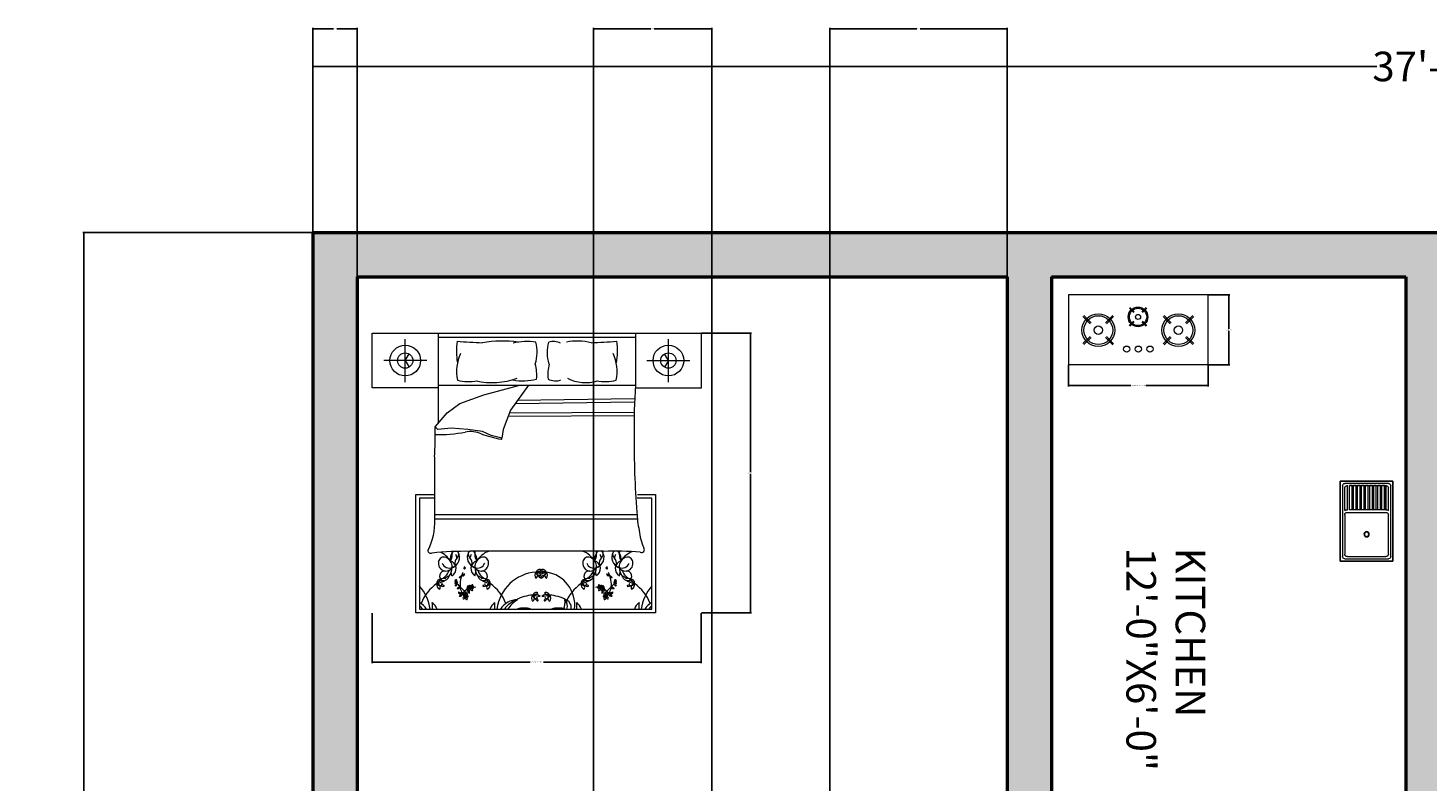
# Model space of a CAD drawing. Units: inches. Extents: x -17 to 536, y -817 to 53.
# Tile 6 of 9: x -17 to 268, y -100 to 53. Entities that reach past the tile are written whole.
import ezdxf

# ---------------------------------------------------------------- set-up
doc = ezdxf.new("R2010")
doc.units = ezdxf.units.IN
doc.header["$MEASUREMENT"] = 0
for name, color, linetype, lineweight in [('A-ANNO-DIMS', 2, 'Continuous', 18), ('A-AREA-IDEN', 7, 'Continuous', 18), ('A-EQPM', 8, 'Continuous', 18), ('A-FLOR-FIXT', 9, 'Continuous', 18), ('A-FURN', 8, 'Continuous', 13), ('A-WALL', 7, 'Continuous', 50), ('A-WALL-PATT', 22, 'Continuous', 13)]:
    doc.layers.add(name, color=color, linetype=linetype, lineweight=lineweight)
doc.styles.get("Standard").update_dxf_attribs({"font": 'arial.ttf'})
doc.dimstyles.get("Standard").update_dxf_attribs({"dimtxt": 0.18, "dimasz": 0.18, "dimexe": 0.18, "dimexo": 0.0625, "dimgap": 0.09, "dimtad": 0, "dimtih": 1, "dimtoh": 1, "dimdec": 0, "dimzin": 0, "dimdsep": 46, "dimlunit": 3, "dimtxsty": 'Standard', "dimcen": 0.09, "dimadec": 0, "dimazin": 0, "dimtfac": 1, "dimtdec": 0, "dimtofl": 0, "dimtmove": 0, "dimatfit": 3, "dimfxl": 1, "dimtolj": 1, "dimtzin": 0, "dimarcsym": 0})

# ---------------------------------------------------------------- blocks, each defined once
blk = doc.blocks.new('*D1')
at = {"layer": 'A-ANNO-DIMS', "color": 0, "lineweight": -2, "transparency": 16777216}
for p, q in [((41.37, 11.61), (41.37, 45.45)), ((41.55, 45.27), (257.47, 45.27)), ((494.19, 45.27), (278.26, 45.27)), ((494.37, 11.61), (494.37, 45.45))]:
    blk.add_line(p, q, dxfattribs=at)
at = {"layer": 'A-ANNO-DIMS', "color": 0, "transparency": 16777216}
for points in [[(41.55, 45.3), (41.55, 45.24), (41.37, 45.27)], [(494.19, 45.3), (494.19, 45.24), (494.37, 45.27)]]:
    blk.add_solid(points, dxfattribs=at)
at = {"layer": 'Defpoints', "color": 0, "transparency": 16777216}
for p in [(494.37, 45.27), (41.37, 11.55), (494.37, 11.55)]:
    blk.add_point(p, dxfattribs=at)
at = {"layer": 'A-ANNO-DIMS', "color": 0, "transparency": 16777216, "insert": (267.87, 45.27), "char_height": 6, "attachment_point": 5}
blk.add_mtext('\\A1;37\'-9"', dxfattribs=at)
blk = doc.blocks.new('*D2')
at = {"layer": 'A-ANNO-DIMS', "color": 0, "lineweight": -2, "transparency": 16777216}
for p, q in [((41.3, 11.55), (-5.38, 11.55)), ((-5.2, 11.37), (-5.2, -378.8)), ((-5.2, -775.27), (-5.2, -385.1)), ((41.3, -775.45), (-5.38, -775.45))]:
    blk.add_line(p, q, dxfattribs=at)
at = {"layer": 'A-ANNO-DIMS', "color": 0, "transparency": 16777216}
for points in [[(-5.23, 11.37), (-5.17, 11.37), (-5.2, 11.55)], [(-5.23, -775.27), (-5.17, -775.27), (-5.2, -775.45)]]:
    blk.add_solid(points, dxfattribs=at)
at = {"layer": 'Defpoints', "color": 0, "transparency": 16777216}
for p in [(41.37, 11.55), (-5.2, -775.45), (41.37, -775.45)]:
    blk.add_point(p, dxfattribs=at)
at = {"layer": 'A-ANNO-DIMS', "color": 0, "transparency": 16777216, "insert": (-5.2, -381.95), "char_height": 6, "attachment_point": 5}
blk.add_mtext('\\A1;65\'-7"', dxfattribs=at)
blk = doc.blocks.new('М12 540х820')
for p, q in [((0, 540), (-820, 540)), ((-820, 540), (-820, 0)), ((-798, 495), (-798, 45)), ((-45, 517), (-775, 517)), ((-775, 468), (-775, 72)), ((-348, 495), (-748, 495)), ((-320, 468), (-320, 72)), ((-302, 495), (-65, 495)), ((-294, 468), (-294, 472)), ((-294, 468), (-45, 468)), ((-294, 447), (-45, 447)), ((-294, 420), (-294, 447)), ((-45, 470), (-45, 468)), ((-45, 420), (-45, 447)), ((-22, 45), (-22, 495)), ((0, 0), (0, 540)), ((-294, 420), (-45, 420)), ((-294, 405), (-45, 405)), ((-294, 378), (-294, 405)), ((-294, 378), (-45, 378)), ((-294, 336), (-294, 363)), ((-294, 363), (-45, 363)), ((-294, 336), (-45, 336)), ((-294, 295), (-294, 322)), ((-294, 322), (-45, 322)), ((-294, 295), (-45, 295)), ((-45, 378), (-45, 405)), ((-45, 336), (-45, 363)), ((-45, 295), (-45, 322)), ((-294, 253), (-294, 280)), ((-294, 280), (-45, 280)), ((-294, 253), (-45, 253)), ((-294, 211), (-294, 238)), ((-294, 238), (-45, 238)), ((-294, 211), (-45, 211)), ((-294, 170), (-294, 197)), ((-294, 197), (-45, 197)), ((-294, 170), (-45, 170)), ((-294, 128), (-294, 155)), ((-294, 155), (-45, 155)), ((-45, 253), (-45, 280)), ((-45, 211), (-45, 238)), ((-45, 170), (-45, 197)), ((-45, 128), (-45, 155)), ((-820, 0), (0, 0)), ((-775, 22), (-45, 22)), ((-748, 45), (-348, 45)), ((-302, 45), (-65, 45)), ((-294, 128), (-45, 128)), ((-294, 114), (-45, 114)), ((-294, 87), (-294, 114)), ((-294, 87), (-45, 87)), ((-294, 72), (-45, 72)), ((-45, 87), (-45, 114)), ((-45, 70), (-45, 72))]:
    blk.add_line(p, q)
at = {"ltscale": 0.06}
for p, q in [((-820, 0), (-820, 540)), ((-820, 540), (0, 540)), ((-294, 447), (-45, 447)), ((-294, 405), (-294, 447)), ((-45, 447), (-45, 420)), ((0, 540), (0, 537)), ((0, 537), (0, 0)), ((-294, 363), (-294, 405)), ((-294, 322), (-294, 363)), ((-294, 280), (-294, 322)), ((-45, 420), (-45, 378)), ((-45, 378), (-45, 336)), ((-45, 336), (-45, 295)), ((-45, 295), (-45, 253)), ((-294, 238), (-294, 280)), ((-294, 197), (-294, 238)), ((-294, 155), (-294, 197)), ((-294, 114), (-294, 155)), ((-45, 253), (-45, 211)), ((-45, 211), (-45, 170)), ((-45, 170), (-45, 128)), ((0, 0), (-820, 0)), ((-294, 72), (-294, 114)), ((-45, 72), (-294, 72)), ((-45, 128), (-45, 87)), ((-45, 87), (-45, 72))]:
    blk.add_line(p, q, dxfattribs=at)
at = {"extrusion": (0, 0, -1)}
for centre, major_axis, start_param, end_param in [((-775, 495), (-15.9, 15.9), -0.785398, 0.785398), ((-775, 495), (-15.9, 15.9), -0.785398, 0.785398), ((-748, 468), (-19.1, -19.1), 0.785398, 2.356194), ((-748, 468), (-19.1, -19.1), 0.785398, 2.356194), ((-348, 468), (-19.1, 19.1), 0.785398, 2.356194), ((-348, 468), (-19.1, 19.1), 0.785398, 2.356194), ((-343, 468), (-35, 35), 1.779263, 2.356194), ((-343, 468), (-35, 35), 1.779263, 2.356192), ((-343, 468), (-35, 35), 2.356192, 2.356194), ((-72, 469), (-19.3, 19.3), 1.0328, 2.38382), ((-72, 469), (-19.3, 19.3), 1.0328, 1.064673), ((-72, 469), (-19.3, 19.3), 1.064673, 2.328569), ((-45, 495), (-15.9, -15.9), 2.356194, 3.926991), ((-45, 495), (-15.9, -15.9), 2.356194, 3.926991), ((-72, 469), (-19.3, 19.3), 2.328569, 2.38382), ((-545, 270), (-19.1, -19.1), 3.926991, 10.210176), ((-545, 270), (-19.1, -19.1), 3.926991, 10.210176), ((-545, 270), (-15.9, -15.9), 3.926991, 10.210176), ((-545, 270), (-15.9, -15.9), 3.926991, 10.210176), ((-775, 45), (-15.9, -15.9), 5.497787, 7.068583), ((-775, 45), (-15.9, -15.9), 5.497787, 7.068583), ((-748, 72), (-19.1, 19.1), 3.926991, 5.497787), ((-748, 72), (-19.1, 19.1), 3.926991, 5.497787), ((-348, 72), (-19.1, -19.1), 3.926991, 5.497787), ((-348, 72), (-19.1, -19.1), 3.926991, 5.497787), ((-343, 72), (-35, -35), 3.926991, 4.503922), ((-343, 72), (-35, -35), 3.926991, 4.503922), ((-72, 71), (-19.3, -19.3), 3.899365, 5.250385), ((-72, 71), (-19.3, -19.3), 5.218512, 5.250385), ((-72, 71), (-19.3, -19.3), 3.954617, 5.218512), ((-72, 71), (-19.3, -19.3), 3.899365, 3.954617), ((-45, 45), (-15.9, 15.9), 2.356194, 3.926991), ((-45, 45), (-15.9, 15.9), 2.356194, 3.926991)]:
    blk.add_ellipse(centre, major_axis=major_axis, ratio=1, start_param=start_param, end_param=end_param, dxfattribs=at)
blk = doc.blocks.new('BED-WITH-NIGHTSTANDS-COMPACT')
for p, q in [((0, 56.83), (66.83, 56.83)), ((6.68, 46.9), (6.68, 55.63)), ((13.37, 56.83), (13.37, 38.49)), ((53.46, 55.97), (13.37, 55.97)), ((60.14, 46.9), (60.14, 55.63)), ((11.05, 51.26), (2.32, 51.26)), ((55.78, 51.26), (64.51, 51.26)), ((13.37, 46.27), (53.46, 46.27)), ((22.65, 44.28), (29.94, 46.27)), ((31.72, 46.27), (28.06, 41.17)), ((17.78, 42.53), (22.65, 44.28)), ((53.26, 42.81), (28.99, 42.47)), ((53.28, 43.49), (29.49, 43.16)), ((12.77, 37.79), (15.2, 40.63)), ((15.2, 40.63), (17.78, 42.53)), ((28.06, 41.17), (26.57, 37.25)), ((53.23, 40.02), (27.58, 39.91)), ((53.22, 40.7), (27.85, 40.6)), ((13.31, 37.25), (12.77, 37.79)), ((16.02, 37.52), (13.31, 37.25)), ((19.4, 37.25), (16.02, 37.52)), ((22.38, 36.85), (19.4, 37.25)), ((26.57, 37.25), (26.3, 35.49)), ((24.14, 36.03), (22.38, 36.85)), ((26.3, 35.49), (24.14, 36.03)), ((8.82, 24.07), (12.6, 24.07)), ((8.82, 0), (8.82, 24.07)), ((12.6, 23.3), (9.59, 23.3)), ((9.59, 23.3), (9.59, 0.77)), ((56.77, 23.3), (53.82, 23.3)), ((53.83, 24.07), (57.54, 24.07)), ((56.77, 0.77), (56.77, 23.3)), ((57.54, 24.07), (57.54, 0)), ((53.77, 19.9), (12.6, 19.9)), ((53.83, 19.07), (12.6, 19.07)), ((46.98, 12.51), (19.85, 12.51)), ((16.18, 7.55), (16.03, 8.3)), ((20.85, 7.55), (21, 8.3)), ((45.51, 7.55), (45.36, 8.3)), ((50.18, 7.55), (50.33, 8.3)), ((9.59, 0.77), (56.77, 0.77)), ((57.54, 0), (8.82, 0))]:
    blk.add_line(p, q)
for points in [[(13.37, 45.69), (0, 45.69), (0, 56.83)], [(53.46, 56.83), (53.46, 45.69), (66.83, 45.69), (66.83, 56.83)], [(6.68, 51.26), (7.46, 52.61)], [(6.68, 51.26), (7.46, 49.91)], [(60.14, 51.26), (59.36, 52.61)], [(60.14, 51.26), (59.36, 49.91)]]:
    blk.add_lwpolyline(points)
for points in [[(17.2, 55.17, 0.074897), (17.28, 50.8, -0.472817)], [(33.1, 50.56, 0.14099), (33.23, 55.01, 0.235245)], [(35.95, 50.56, -0.14099), (35.82, 55.01, -0.235245)], [(49.62, 55.17, -0.074897), (49.54, 50.8, 0.472817)], [(12.63, 31.67, 0.001242), (12.6, 18.99, -0.127202), (11.26, 12.67)], [(53.75, 20.43, 0.056112), (54.23, 16.75, 0.095341), (55.17, 13.21)]]:
    blk.add_lwpolyline(points, format="xyb")
for centre, radius in [((6.68, 51.26), 3.12), ((60.14, 51.26), 3.12), ((6.68, 51.26), 1.56), ((60.14, 51.26), 1.56), ((18.93, 3.33), 0.17), ((20.04, 5.13), 0.17), ((46.32, 5.13), 0.17), ((47.43, 3.33), 0.17)]:
    blk.add_circle(centre, radius)
for centre, radius, start, end in [((54.04, 691.14), 637.04, 266.68521, 267.14978), ((26.36, 30.98), 24.24, 82.2196, 99.497), ((31.48, 43.23), 11.91, 81.5249, 103.96), ((36.74, 51.83), 3.31, 63.3437, 106.1026), ((41.69, 43.47), 11.75, 76.3427, 101.1841), ((12.79, 691.14), 637.04, 272.85022, 273.31479), ((25.72, 49.05), 8.61, 155.1316, 191.7583), ((41.11, 49.05), 8.61, 348.2417, 24.8684), ((25.22, 48.32), 8.19, 354.0129, 15.8293), ((43.83, 48.32), 8.19, 164.1707, 185.9871), ((19.59, 55.95), 8.96, 255.1039, 281.0369), ((24.3, 62.31), 15.53, 258.0397, 289.2615), ((30.59, 58.92), 11.78, 259.8617, 283.6238), ((37.18, 50.68), 3.54, 245.0183, 288.5407), ((43.37, 55.29), 8.51, 243.8761, 286.1746), ((47.24, 55.95), 8.96, 258.9631, 284.8961), ((173.26, 38.1), 120.08, 176.1, 180.9282), ((-48.51, 36.13), 61.3, 355.8294, 1.553), ((13.91, 61.46), 25.22, 267.4519, 281.3392), ((19.94, 31.39), 5.44, 66.2616, 101.3392), ((30.94, 60.75), 25.92, 250.1194, 259.3383), ((26.15, 35.44), 0.161, 268.8623, 19.7536), ((209.82, 33.74), 156.63, 179.1145, 184.8735), ((11.87, 12.72), 0.617, 183.98, 297.3412), ((19.05, -57.06), 69.57, 89.3433, 95.6887), ((11.61, 7.8), 5.06, 33.6671, 63.2997), ((18.39, 10.81), 2.58, 145.785, 184.7304), ((13.47, 12.01), 2.77, 328.8218, 9.1554), ((16.89, 11.77), 0.805, 120.0293, 142.325), ((15.61, 11.29), 2.13, 289.2822, 29.1751), ((15.29, 10.91), 1.92, 7.436, 29.9149), ((16.55, 11.93), 1, 311.5653, 23.8354), ((16.89, 11.77), 0.805, 44.4517, 63.558), ((21.42, 11.29), 2.13, 150.8249, 250.7178), ((20.48, 11.93), 1, 156.1646, 228.4347), ((20.14, 11.77), 0.805, 113.229, 135.5483), ((21.74, 10.91), 1.92, 150.0851, 172.564), ((20.14, 11.77), 0.805, 37.675, 66.7144), ((18.64, 10.81), 2.58, 355.2696, 34.215), ((23.57, 12.01), 2.77, 169.7133, 211.1782), ((25.42, 7.8), 5.06, 111.4941, 146.3329), ((40.94, 7.8), 5.06, 33.6671, 68.5059), ((47.72, 10.81), 2.58, 145.785, 184.7304), ((42.79, 12.01), 2.77, 328.8218, 10.2867), ((46.22, 11.77), 0.805, 113.2856, 142.325), ((44.94, 11.29), 2.13, 289.2822, 29.1751), ((44.62, 10.91), 1.92, 7.436, 29.9149), ((46.22, 11.77), 0.805, 44.4517, 66.7144), ((45.88, 11.93), 1, 311.5653, 23.8354), ((49.03, -52.49), 65.03, 85.2402, 91.8035), ((50.75, 11.29), 2.13, 150.8249, 250.7178), ((49.81, 11.93), 1, 156.1646, 228.4347), ((49.47, 11.77), 0.805, 106.6343, 135.5483), ((51.07, 10.91), 1.92, 150.0851, 172.564), ((49.47, 11.77), 0.805, 37.675, 72.5814), ((47.97, 10.81), 2.58, 355.2696, 34.215), ((52.9, 12.01), 2.77, 169.249, 211.1782), ((54.75, 7.8), 5.06, 113.6453, 146.3329), ((54.66, 12.87), 0.609, 246.5219, 33.8264), ((15.02, 10.07), 1.6, 174.9449, 262.8857), ((14.56, 10.23), 1.13, 84.4856, 181.0538), ((15.65, 10.67), 1.55, 201.5819, 291.4221), ((12.66, 9.7), 3.15, 301.2614, 341.7045), ((14.21, 9.39), 2.01, 355.2933, 76.921), ((14.74, 10.42), 1.94, 272.3591, 324.0401), ((12.63, 9.45), 3.59, 326.2883, 356.5076), ((15.35, 8.99), 1.66, 299.9085, 73.1337), ((18.39, 10.81), 2.58, 212.7011, 216.3445), ((16.4, 9.69), 0.415, 257.3041, 15.1471), ((18.13, 10.15), 1.37, 131.5653, 195.1471), ((18.71, 9.06), 0.129, 102.7051, 280.4384), ((18.69, 9.14), 0.209, 280.4384, 100.4136), ((18.9, 10.15), 1.37, 344.8529, 48.4347), ((21.68, 8.99), 1.66, 106.8663, 240.0915), ((20.63, 9.69), 0.415, 164.8529, 282.6959), ((18.64, 10.81), 2.58, 323.6555, 327.2989), ((22.29, 10.42), 1.94, 215.9599, 267.6409), ((22.82, 9.39), 2.01, 103.079, 184.7067), ((21.38, 10.67), 1.55, 248.5779, 338.4181), ((24.4, 9.45), 3.59, 183.4924, 213.7117), ((24.37, 9.7), 3.15, 198.2955, 238.7386), ((22.01, 10.07), 1.6, 277.1143, 5.0551), ((22.47, 10.23), 1.13, 358.9462, 95.5144), ((33.95, 8.1), 0.723, 63.0274, 163.8037), ((33.22, 9.79), 1.49, 271.4585, 315.3727), ((34.64, 8.1), 0.723, 16.1963, 116.9726), ((35.37, 9.79), 1.49, 224.6273, 268.5415), ((44.35, 10.07), 1.6, 174.9449, 262.8857), ((43.89, 10.23), 1.13, 84.4856, 181.0538), ((44.98, 10.67), 1.55, 201.5819, 291.4221), ((41.99, 9.7), 3.15, 301.2614, 341.7045), ((43.54, 9.39), 2.01, 355.2933, 76.921), ((44.07, 10.42), 1.94, 272.3591, 324.0401), ((41.96, 9.45), 3.59, 326.2883, 356.5076), ((44.68, 8.99), 1.66, 299.9085, 73.1337), ((47.72, 10.81), 2.58, 212.7011, 216.3445), ((45.73, 9.69), 0.415, 257.3041, 15.1471), ((47.46, 10.15), 1.37, 131.5653, 195.1471), ((47.67, 9.14), 0.209, 79.5864, 259.5616), ((47.65, 9.06), 0.129, 259.5616, 77.2949), ((48.23, 10.15), 1.37, 344.8529, 48.4347), ((51.01, 8.99), 1.66, 106.8663, 240.0915), ((49.96, 9.69), 0.415, 164.8529, 282.6959), ((47.97, 10.81), 2.58, 323.6555, 327.2989), ((51.62, 10.42), 1.94, 215.9599, 267.6409), ((52.15, 9.39), 2.01, 103.079, 184.7067), ((50.71, 10.67), 1.55, 248.5779, 338.4181), ((53.73, 9.45), 3.59, 183.4924, 213.7117), ((53.7, 9.7), 3.15, 198.2955, 238.7386), ((51.34, 10.07), 1.6, 277.1143, 5.0551), ((51.8, 10.23), 1.13, 358.9462, 95.5144), ((18.03, -1.26), 8.73, 124.3865, 158.5908), ((13.8, 6.11), 0.723, 92.9516, 193.728), ((14.05, 5.73), 0.968, 167.7115, 249.0387), ((12.32, 7.21), 1.49, 301.3827, 345.2969), ((14.22, 5.13), 1.38, 75.4653, 144.2343), ((11.78, 11.9), 6.1, 282.5173, 297.1824), ((13.08, 5.21), 0.729, 328.4633, 88.2869), ((14.55, 7.6), 2.21, 228.8402, 267.9352), ((13.73, 6.27), 0.714, 207.6827, 313.7762), ((14.65, 7.5), 1, 80.264, 250.8688), ((14.45, 6.41), 0.615, 63.9755, 143.2681), ((14.16, 5.82), 0.0944, 313.7762, 249.7183), ((14.41, 7.8), 1.25, 265.969, 344.3045), ((15.76, 6.13), 1.33, 96.1662, 141.5825), ((16.98, 6.4), 0.284, 101.5637, 142.6358), ((16.74, 6.14), 0.17, 273.2768, 86.7232), ((16.94, 6.3), 0.163, 91.1081, 181.8675), ((17.28, 6.2), 0.517, 203.4276, 227.6104), ((17.11, 5.97), 0.352, 80.3487, 133.6538), ((17.05, 6.26), 0.278, 229.7889, 317.6792), ((16.75, 6.63), 0.409, 288.7263, 352.5032), ((16.74, 5.67), 0.395, 355.053, 68.3618), ((17.05, 5.61), 0.557, 83.0852, 105.7171), ((17.03, 6.61), 0.131, 345.2356, 144.9248), ((13.19, 0.99), 6.35, 43.1541, 52.0459), ((17.15, 6.18), 0.147, 317.6792, 80.3487), ((17.97, 7.07), 0.351, 101.3256, 154.4621), ((17.46, 8.26), 1.06, 280.2588, 300.656), ((17.71, 9.1), 1.88, 268.3264, 277.1302), ((23.34, 5.69), 5.53, 163.5842, 183.8277), ((17.24, 8.26), 1.07, 308.2101, 316.3071), ((17.9, 7.55), 0.321, 278.3432, 4.2869), ((17.72, 7.83), 0.56, 300.656, 332.6341), ((18.14, 7.46), 0.136, 55.7657, 157.4417), ((23.34, 5.69), 5.53, 153.0032, 159.8941), ((18.35, 7.59), 0.136, 84.3784, 186.0543), ((18.22, 8.13), 0.56, 269.1859, 301.164), ((18.39, 7.84), 0.321, 237.5332, 323.4768), ((18.08, 8.76), 1.07, 285.5129, 293.6099), ((17.97, 8.56), 1.06, 301.164, 321.5612), ((18.78, 7.55), 0.351, 87.3579, 140.4944), ((17.11, 8.74), 1.88, 324.6898, 333.4936), ((20.33, 5.59), 0.131, 345.2356, 144.9248), ((21.27, 6.13), 1.33, 38.4175, 83.8338), ((22.62, 7.8), 1.25, 195.6955, 274.031), ((22.38, 7.5), 1, 289.1312, 99.736), ((22.59, 6.41), 0.615, 36.7319, 116.0245), ((22.81, 5.13), 1.38, 35.7657, 104.5347), ((25.25, 11.9), 6.1, 242.8176, 257.4827), ((22.48, 7.6), 2.21, 272.0648, 311.1598), ((23.3, 6.27), 0.714, 226.2238, 332.3173), ((22.88, 5.86), 0.0569, 290.2667, 226.2271), ((23.95, 5.21), 0.729, 91.7131, 211.5367), ((23.23, 6.11), 0.723, 346.272, 87.0484), ((24.71, 7.21), 1.49, 194.7031, 238.6173), ((22.99, 5.73), 0.968, 290.9613, 12.2885), ((19, -1.26), 8.73, 21.4092, 55.6135), ((33.93, -0.4), 8.73, 94.4623, 172.255), ((33.97, 7.65), 0.968, 137.7873, 219.1145), ((32.87, 7.68), 0.729, 298.5391, 58.3627), ((33.82, 7.04), 1.38, 45.5411, 114.3101), ((35.08, 14.12), 6.1, 252.593, 267.2582), ((33.97, 8.27), 0.714, 177.7585, 283.852), ((35.34, 9.01), 2.21, 198.9159, 238.011), ((34.77, 7.04), 1.38, 65.6899, 134.4589), ((33.51, 14.12), 6.1, 272.7418, 287.407), ((34.12, 7.67), 0.0944, 283.852, 219.9245), ((34.23, 7.23), 0.108, 238.011, 71.5592), ((34.25, 7.29), 0.0526, 71.5592, 188.0167), ((34.36, 7.23), 0.108, 108.4408, 301.989), ((34.34, 7.29), 0.0526, 351.9833, 108.4408), ((34.46, 7.71), 0.0569, 320.1909, 256.0209), ((33.25, 9.01), 2.21, 301.989, 341.0841), ((34.62, 8.27), 0.714, 256.148, 2.2415), ((35.72, 7.68), 0.729, 121.6373, 241.4609), ((34.62, 7.65), 0.968, 320.8855, 42.2127), ((34.37, 1.61), 6.75, 352.8636, 81.8197), ((47.36, -1.26), 8.73, 124.3865, 158.5908), ((43.13, 6.11), 0.723, 92.9516, 193.728), ((43.37, 5.73), 0.968, 167.7115, 249.0387), ((41.65, 7.21), 1.49, 301.3827, 345.2969), ((43.55, 5.13), 1.38, 75.4653, 144.2343), ((41.11, 11.9), 6.1, 282.5173, 297.1824), ((43.06, 6.27), 0.714, 207.6827, 313.7762), ((43.88, 7.6), 2.21, 228.8402, 267.9352), ((42.41, 5.21), 0.729, 328.4633, 88.2869), ((43.98, 7.5), 1, 80.264, 250.8688), ((43.77, 6.41), 0.615, 63.9755, 143.2681), ((43.49, 5.82), 0.0944, 313.7762, 249.7183), ((43.74, 7.8), 1.25, 265.969, 344.3045), ((45.09, 6.13), 1.33, 96.1662, 141.5825), ((46.03, 5.59), 0.131, 35.0752, 194.7644), ((48.39, 8.56), 1.06, 218.4388, 238.836), ((47.58, 7.55), 0.351, 39.5056, 92.6421), ((49.25, 8.74), 1.88, 206.5064, 215.3102), ((47.97, 7.84), 0.321, 216.5232, 302.4668), ((48.28, 8.76), 1.07, 246.3901, 254.4871), ((48.14, 8.13), 0.56, 238.836, 270.8141), ((43.02, 5.69), 5.53, 20.1059, 26.9968), ((48.01, 7.59), 0.136, 353.9457, 95.6216), ((48.47, 7.55), 0.321, 175.7131, 261.6568), ((48.22, 7.46), 0.136, 22.5583, 124.2343), ((48.64, 7.83), 0.56, 207.3659, 239.344), ((43.02, 5.69), 5.53, 356.1723, 16.4158), ((49.12, 8.26), 1.07, 223.6929, 231.7899), ((48.9, 8.26), 1.06, 239.344, 259.7412), ((48.65, 9.1), 1.88, 262.8698, 271.6736), ((48.39, 7.07), 0.351, 25.5379, 78.6744), ((53.17, 0.99), 6.35, 127.9541, 136.8459), ((49.21, 6.18), 0.147, 99.6513, 222.3208), ((49.31, 6.26), 0.278, 222.3208, 310.2111), ((49.25, 5.97), 0.352, 46.3462, 99.6513), ((49.33, 6.61), 0.131, 35.0752, 194.7644), ((49.61, 6.63), 0.409, 187.4968, 251.2737), ((49.62, 5.67), 0.395, 111.6382, 184.947), ((49.31, 5.61), 0.557, 74.2829, 96.9148), ((49.42, 6.3), 0.163, 358.1325, 88.8919), ((49.08, 6.2), 0.517, 312.3896, 336.5724), ((49.38, 6.4), 0.284, 37.3642, 78.4363), ((49.62, 6.14), 0.17, 93.2768, 266.7232), ((51.95, 7.8), 1.25, 195.6955, 274.031), ((50.6, 6.13), 1.33, 38.4175, 83.8338), ((51.71, 7.5), 1, 289.1312, 99.736), ((51.92, 6.41), 0.615, 36.7319, 116.0245), ((52.14, 5.13), 1.38, 35.7657, 104.5347), ((54.58, 11.9), 6.1, 242.8176, 257.4827), ((51.81, 7.6), 2.21, 272.0648, 311.1598), ((52.63, 6.27), 0.714, 226.2238, 332.3173), ((52.21, 5.86), 0.0569, 290.2667, 226.2271), ((53.28, 5.21), 0.729, 91.7131, 211.5367), ((54.04, 7.21), 1.49, 194.7031, 238.6173), ((52.56, 6.11), 0.723, 346.272, 87.0484), ((52.32, 5.73), 0.968, 290.9613, 12.2885), ((48.33, -1.26), 8.73, 21.4092, 55.6135), ((3.1, -0.4), 8.73, 7.745, 41.8856), ((14.47, 5.56), 0.0526, 101.4834, 217.9409), ((14.48, 5.5), 0.108, 267.9352, 101.4834), ((16.97, 5.82), 0.281, 217.7621, 259.0403), ((17, 5.65), 0.131, 232.4737, 355.053), ((17.57, 4.82), 0.351, 101.3256, 154.4621), ((17.07, 6.01), 1.06, 280.2588, 300.656), ((17.31, 6.85), 1.88, 268.3264, 277.1302), ((16.84, 6.01), 1.07, 308.2101, 316.3071), ((17.69, 4.2), 0.19, 146.8636, 236.9021), ((20.37, 8.39), 4.97, 235.1882, 238.8844), ((18.02, 4.48), 0.514, 199.4799, 267.6828), ((17.5, 5.3), 0.321, 278.3432, 4.2869), ((17.96, 4.28), 0.443, 212.8155, 277.3992), ((17.74, 5.21), 0.136, 55.7657, 157.4417), ((17.32, 5.58), 0.56, 300.656, 332.6341), ((17.7, 3.99), 0.514, 266.9701, 338.2913), ((14.99, 7.66), 4.97, 302.6784, 306.3746), ((17.83, 3.58), 0.19, 214.3538, 304.3923), ((17.9, 4.3), 0.197, 238.8844, 314.2646), ((20.58, 5.56), 2.77, 184.756, 209.2041), ((24.58, 11.46), 9.13, 222.2412, 232.1744), ((17.86, 3.86), 0.443, 280.3057, 17.1958), ((17.82, 3.81), 0.197, 306.3746, 21.7548), ((18.14, 3.94), 0.148, 19.3605, 201.7548), ((18.14, 4.05), 0.148, 311.8703, 134.2646), ((20.93, 2.7), 2.96, 153.7819, 158.2913), ((18.57, 4.73), 0.776, 247.2305, 319.0635), ((18.32, 4.47), 0.457, 264.4544, 310.6188), ((20.58, 5.56), 2.77, 214.0033, 222.4917), ((18.65, 4.28), 0.472, 218.3208, 298.8162), ((20.87, 1.87), 3.33, 120.544, 139.818), ((18.57, 3.01), 0.169, 148.0499, 225.6268), ((18.88, 2.82), 0.537, 104.7558, 148.0499), ((18.58, 3.2), 0.336, 247.4086, 351.4386), ((18.74, 3.57), 0.232, 126.1046, 271.4281), ((18.71, 3.63), 0.167, 353.7526, 131.7054), ((18.97, 3.7), 0.549, 70.0041, 130.6188), ((18.68, 3.19), 0.113, 262.906, 7.132), ((18.56, 3.44), 0.234, 0.0645, 61.1507), ((18.61, 3.64), 0.268, 311.8413, 355.7877), ((18.62, 4.37), 0.564, 297.7043, 344.3516), ((19.16, 3.6), 0.284, 101.5637, 176.365), ((19.16, 3.02), 0.281, 151.2196, 259.0403), ((19.13, 3.49), 0.163, 91.1081, 181.8675), ((19.46, 3.39), 0.517, 203.4276, 227.6104), ((19.3, 3.17), 0.352, 80.3487, 133.6538), ((19.24, 3.46), 0.278, 229.7889, 317.6792), ((18.94, 3.82), 0.409, 288.7263, 352.5032), ((18.92, 2.87), 0.395, 355.053, 68.3618), ((19.23, 2.8), 0.557, 83.0852, 105.7171), ((19.21, 3.8), 0.131, 345.2356, 144.9248), ((18.74, 5.38), 0.776, 304.5369, 16.3699), ((19.15, 5.21), 0.472, 272.8499, 356.1226), ((18.82, 5.02), 0.457, 321.7607, 7.9252), ((18.92, 4.37), 0.457, 8.7227, 54.8872), ((18.94, 4), 0.776, 0.278, 72.111), ((19.82, 5.16), 0.549, 127.3105, 187.9252), ((19.29, 4.29), 0.472, 20.5253, 88.5375), ((19.33, 3.37), 0.147, 317.6792, 80.3487), ((19.91, 4.52), 0.549, 188.7227, 249.3375), ((19.06, 5.22), 0.564, 355.0106, 41.658), ((19.68, 4.81), 0.169, 148.0499, 225.6268), ((20.87, 1.87), 3.33, 113.0501, 113.8477), ((20, 4.61), 0.537, 104.7558, 148.0499), ((19.69, 5), 0.336, 247.4086, 351.4386), ((19.85, 5.36), 0.232, 126.1046, 271.4281), ((19.83, 5.43), 0.167, 353.7526, 131.7054), ((19.2, 4.25), 0.564, 334.9899, 21.6373), ((19.67, 5.23), 0.234, 0.0645, 61.1507), ((19.79, 4.98), 0.113, 262.906, 7.132), ((19.73, 5.43), 0.268, 311.8413, 355.7877), ((20.28, 5.39), 0.284, 101.5637, 176.365), ((20.27, 4.81), 0.281, 151.2196, 259.0403), ((20.24, 5.29), 0.163, 91.1081, 181.8675), ((20.58, 5.19), 0.517, 203.4276, 227.6104), ((20.41, 4.96), 0.352, 80.3487, 133.6538), ((20.35, 5.25), 0.278, 229.7889, 317.6792), ((20.05, 5.61), 0.409, 288.7263, 352.5032), ((20.04, 4.66), 0.395, 355.053, 68.3618), ((20.35, 4.6), 0.557, 83.0852, 105.7171), ((20.3, 4.64), 0.131, 232.4737, 355.053), ((20.45, 5.16), 0.147, 317.6792, 80.3487), ((20.87, 1.87), 3.33, 87.1071, 94.7585), ((22.55, 5.5), 0.108, 78.5166, 272.0648), ((22.57, 5.56), 0.0526, 322.0591, 78.5166), ((33.26, -5.08), 8.73, 94.4623, 117.4146), ((33.3, 2.97), 0.968, 137.7873, 219.1145), ((32.2, 3), 0.729, 298.5391, 58.3627), ((33.28, 3.42), 0.723, 63.0274, 163.8037), ((32.55, 5.11), 1.49, 271.4585, 315.3727), ((33.15, 2.37), 1.38, 45.5411, 114.3101), ((34.67, 4.34), 2.21, 198.9159, 238.011), ((34.41, 9.45), 6.1, 252.593, 267.2582), ((33.3, 3.6), 0.714, 177.7585, 283.852), ((33.45, 2.99), 0.0944, 283.852, 219.9245), ((35.43, 2.37), 1.38, 65.6899, 134.4589), ((34.18, 9.45), 6.1, 272.7418, 287.407), ((35.31, 3.42), 0.723, 16.1963, 116.9726), ((36.04, 5.11), 1.49, 224.6273, 268.5415), ((35.13, 3.03), 0.0569, 320.1909, 256.0209), ((33.91, 4.34), 2.21, 301.989, 341.0841), ((35.29, 3.6), 0.714, 256.148, 2.2415), ((36.38, 3), 0.729, 121.6373, 241.4609), ((35.29, 2.97), 0.968, 320.8855, 42.2127), ((35.32, -5.08), 8.73, 62.5854, 85.5377), ((43.79, 5.56), 0.0526, 101.4834, 217.9409), ((43.81, 5.5), 0.108, 267.9352, 101.4834), ((45.49, 1.87), 3.33, 85.2415, 92.8929), ((45.91, 5.16), 0.147, 99.6513, 222.3208), ((46.01, 5.25), 0.278, 222.3208, 310.2111), ((45.95, 4.96), 0.352, 46.3462, 99.6513), ((46.31, 5.61), 0.409, 187.4968, 251.2737), ((46.33, 4.66), 0.395, 111.6382, 184.947), ((46.06, 4.64), 0.131, 184.947, 307.5263), ((46.02, 4.6), 0.557, 74.2829, 96.9148), ((46.12, 5.29), 0.163, 358.1325, 88.8919), ((45.78, 5.19), 0.517, 312.3896, 336.5724), ((46.08, 5.39), 0.284, 3.635, 78.4363), ((46.09, 4.81), 0.281, 280.9597, 28.7804), ((46.67, 5), 0.336, 188.5614, 292.5914), ((46.53, 5.43), 0.167, 48.2946, 186.2474), ((46.63, 5.43), 0.268, 184.2123, 228.1587), ((46.69, 5.23), 0.234, 118.8493, 179.9355), ((46.57, 4.98), 0.113, 172.868, 277.094), ((46.51, 5.36), 0.232, 268.5719, 53.8954), ((46.36, 4.61), 0.537, 31.9501, 75.2442), ((47.16, 4.25), 0.564, 158.3627, 205.0101), ((47.07, 4.29), 0.472, 91.4625, 159.4747), ((47.42, 4), 0.776, 107.889, 179.722), ((46.45, 4.52), 0.549, 290.6625, 351.2773), ((47.3, 5.22), 0.564, 138.342, 184.9894), ((47.21, 5.21), 0.472, 183.8774, 267.1501), ((45.49, 1.87), 3.33, 66.1523, 66.9499), ((46.68, 4.81), 0.169, 314.3732, 31.9501), ((47.62, 5.38), 0.776, 163.6301, 235.4631), ((46.55, 5.16), 0.549, 352.0748, 52.6895), ((47.03, 3.37), 0.147, 99.6513, 222.3208), ((47.12, 3.46), 0.278, 222.3208, 310.2111), ((47.45, 4.37), 0.457, 125.1128, 171.2773), ((47.06, 3.17), 0.352, 46.3462, 99.6513), ((47.15, 3.8), 0.131, 35.0752, 194.7644), ((47.43, 3.82), 0.409, 187.4968, 251.2737), ((47.44, 2.87), 0.395, 111.6382, 184.947), ((47.13, 2.8), 0.557, 74.2829, 96.9148), ((47.54, 5.02), 0.457, 172.0748, 218.2393), ((45.49, 1.87), 3.33, 40.182, 59.456), ((47.39, 3.7), 0.549, 49.3812, 109.9959), ((47.79, 4.73), 0.776, 220.9365, 292.7695), ((47.74, 4.37), 0.564, 195.6484, 242.2957), ((47.23, 3.49), 0.163, 358.1325, 88.8919), ((47.2, 3.6), 0.284, 3.635, 78.4363), ((46.9, 3.39), 0.517, 312.3896, 336.5724), ((47.2, 3.02), 0.281, 280.9597, 28.7804), ((41.78, 11.46), 9.13, 307.8256, 317.7588), ((47.78, 3.2), 0.336, 188.5614, 292.5914), ((47.71, 4.28), 0.472, 241.1838, 321.6792), ((47.65, 3.63), 0.167, 48.2946, 186.2474), ((47.75, 3.64), 0.268, 184.2123, 228.1587), ((47.8, 3.44), 0.234, 118.8493, 179.9355), ((47.68, 3.19), 0.113, 172.868, 277.094), ((47.62, 3.57), 0.232, 268.5719, 53.8954), ((47.48, 2.82), 0.537, 31.9501, 75.2442), ((48.04, 4.47), 0.457, 229.3812, 275.5456), ((45.78, 5.56), 2.77, 317.5083, 325.9967), ((47.79, 3.01), 0.169, 314.3732, 31.9501), ((48.5, 3.86), 0.443, 162.8042, 259.6943), ((48.22, 4.05), 0.148, 45.7354, 228.1297), ((48.22, 3.94), 0.148, 338.2452, 160.6395), ((45.43, 2.7), 2.96, 21.7087, 26.2181), ((48.66, 3.99), 0.514, 201.7087, 273.0299), ((45.78, 5.56), 2.77, 330.7959, 355.244), ((48.46, 4.3), 0.197, 225.7354, 301.1156), ((48.54, 3.81), 0.197, 158.2452, 233.6254), ((48.4, 4.28), 0.443, 262.6008, 327.1845), ((48.35, 4.48), 0.514, 272.3172, 340.5201), ((51.37, 7.66), 4.97, 233.6254, 237.3216), ((48.53, 3.58), 0.19, 235.6077, 325.6462), ((48.62, 5.21), 0.136, 22.5583, 124.2343), ((48.86, 5.3), 0.321, 175.7131, 261.6568), ((49.04, 5.58), 0.56, 207.3659, 239.344), ((45.99, 8.39), 4.97, 301.1156, 304.8118), ((49.52, 6.01), 1.07, 223.6929, 231.7899), ((49.29, 6.01), 1.06, 239.344, 259.7412), ((48.67, 4.2), 0.19, 303.0979, 33.1364), ((49.05, 6.85), 1.88, 262.8698, 271.6736), ((48.79, 4.82), 0.351, 25.5379, 78.6744), ((49.36, 5.65), 0.131, 184.947, 307.5263), ((49.39, 5.82), 0.281, 280.9597, 322.2379), ((51.88, 5.5), 0.108, 78.5166, 272.0648), ((51.9, 5.56), 0.0526, 322.0591, 78.5166), ((63.26, -0.4), 8.73, 138.1144, 172.255), ((7.48, -1.57), 4.25, 33.4617, 60.1116), ((5.95, -2.36), 5.3, 36.3036, 46.4814), ((9.86, -0.59), 3.55, 22.5547, 48.9546), ((0.14, 1.32), 12.07, 357.4081, 3.6519), ((19.19, 2.85), 0.131, 232.4737, 355.053), ((27.17, -0.59), 3.55, 131.0454, 157.4453), ((36.89, 1.32), 12.07, 176.3481, 182.5919), ((29.56, -1.57), 4.25, 91.272, 146.5383), ((31.09, -2.36), 5.3, 107.8504, 143.6964), ((33.87, -3.85), 7.88, 124.0123, 144.053), ((30.82, -3.81), 4.8, 73.5431, 107.0202), ((32.73, -6.29), 7.1, 94.3787, 95.6357), ((36.46, -11.15), 12.68, 109.7217, 109.9028), ((33.56, 2.56), 0.108, 238.011, 71.5592), ((33.58, 2.61), 0.0526, 71.5592, 188.0167), ((35.03, 2.56), 0.108, 108.4408, 301.989), ((35.01, 2.61), 0.0526, 351.9833, 108.4408), ((37.76, -3.81), 4.8, 72.9798, 106.4569), ((35.86, -6.29), 7.1, 84.3643, 85.6213), ((32.13, -11.15), 12.68, 70.0972, 70.2783), ((35.25, 2.23), 3.91, 338.117, 6.6195), ((38.83, 1.14), 1.57, 346.3898, 79.0739), ((37.65, 1.36), 1.98, 342.8609, 41.9049), ((29.47, 1.32), 12.07, 357.4081, 3.6519), ((39.19, -0.59), 3.55, 22.5547, 48.9546), ((47.17, 2.85), 0.131, 184.947, 307.5263), ((56.5, -0.59), 3.55, 131.0454, 157.4453), ((66.22, 1.32), 12.07, 176.3481, 182.5919), ((58.88, -1.57), 4.25, 119.8884, 146.5383), ((60.41, -2.36), 5.3, 133.5186, 143.6964)]:
    blk.add_arc(centre, radius, start, end)
blk = doc.blocks.new('COOKTOP-3-BURNER')
for p, q in [((28.32, 14.16), (0, 14.16)), ((0, 14.16), (0, 0)), ((13.21, 10.58), (12.33, 11.47)), ((13.33, 10.7), (12.44, 11.58)), ((14.86, 10.7), (15.74, 11.58)), ((14.97, 10.58), (15.86, 11.47)), ((28.32, 0), (28.32, 14.16)), ((4.36, 8.28), (2.89, 9.76)), ((4.56, 8.48), (3.08, 9.95)), ((7.48, 8.49), (8.95, 9.98)), ((7.68, 8.3), (9.14, 9.78)), ((13.2, 8.83), (12.31, 7.95)), ((13.32, 8.71), (12.43, 7.83)), ((14.86, 8.71), (15.76, 7.83)), ((14.98, 8.83), (15.87, 7.95)), ((20.64, 8.3), (19.18, 9.78)), ((20.84, 8.49), (19.38, 9.98)), ((23.76, 8.48), (25.24, 9.95)), ((23.96, 8.28), (25.43, 9.76)), ((4.36, 5.74), (2.89, 4.27)), ((7.68, 5.73), (9.14, 4.24)), ((20.64, 5.73), (19.18, 4.24)), ((23.96, 5.74), (25.43, 4.27)), ((4.56, 5.54), (3.08, 4.07)), ((7.48, 5.53), (8.95, 4.05)), ((20.84, 5.53), (19.38, 4.05)), ((23.76, 5.54), (25.24, 4.07)), ((0, 0), (28.32, 0))]:
    blk.add_line(p, q)
for centre, radius in [((14.09, 9.7), 2), ((14.09, 9.7), 1.76), ((6.03, 7.01), 3.33), ((6.03, 7.01), 2.93), ((14.09, 9.7), 0.515), ((22.29, 7.01), 3.33), ((22.29, 7.01), 2.93), ((6.03, 7.01), 0.858), ((22.29, 7.01), 0.858), ((11.8, 3.15), 0.629), ((14.16, 3.15), 0.629), ((16.52, 3.15), 0.629)]:
    blk.add_circle(centre, radius)
blk = doc.blocks.new('*D20')
at = {"layer": 'A-ANNO-DIMS', "color": 0, "lineweight": -2, "transparency": 16777216}
for p, q in [((53.43, -65.79), (53.43, -75.93)), ((120.25, -65.79), (120.25, -75.93)), ((53.61, -75.75), (85.51, -75.75)), ((120.07, -75.75), (88.17, -75.75))]:
    blk.add_line(p, q, dxfattribs=at)
at = {"layer": 'A-ANNO-DIMS', "color": 0, "transparency": 16777216}
for points in [[(53.61, -75.72), (53.61, -75.78), (53.43, -75.75)], [(120.07, -75.72), (120.07, -75.78), (120.25, -75.75)]]:
    blk.add_solid(points, dxfattribs=at)
at = {"layer": 'Defpoints', "color": 0, "transparency": 16777216}
for p in [(53.43, -65.73), (120.25, -65.73), (120.25, -75.75)]:
    blk.add_point(p, dxfattribs=at)
at = {"layer": 'A-ANNO-DIMS', "color": 0, "transparency": 16777216, "insert": (86.84, -75.75), "char_height": 0.18, "attachment_point": 5}
blk.add_mtext('\\A1;BED SET B 5\'-7" TYP.', dxfattribs=at)
blk = doc.blocks.new('*D21')
at = {"layer": 'A-ANNO-DIMS', "color": 0, "lineweight": -2, "transparency": 16777216}
for p, q in [((120.32, -8.9), (130.46, -8.9)), ((130.28, -9.08), (130.28, -37.13)), ((130.28, -65.55), (130.28, -37.49)), ((120.32, -65.73), (130.46, -65.73))]:
    blk.add_line(p, q, dxfattribs=at)
at = {"layer": 'A-ANNO-DIMS', "color": 0, "transparency": 16777216}
for points in [[(130.25, -9.08), (130.31, -9.08), (130.28, -8.9)], [(130.25, -65.55), (130.31, -65.55), (130.28, -65.73)]]:
    blk.add_solid(points, dxfattribs=at)
at = {"layer": 'Defpoints', "color": 0, "transparency": 16777216}
for p in [(120.25, -8.9), (130.28, -8.9), (120.25, -65.73)]:
    blk.add_point(p, dxfattribs=at)
at = {"layer": 'A-ANNO-DIMS', "color": 0, "transparency": 16777216, "insert": (130.28, -37.31), "char_height": 0.18, "attachment_point": 5}
blk.add_mtext('\\A1;4\'-9" TYP.', dxfattribs=at)
blk = doc.blocks.new('*D30')
at = {"layer": 'A-ANNO-DIMS', "color": 0, "lineweight": -2, "transparency": 16777216}
for p, q in [((194.87, -15.37), (194.87, -19.73)), ((223.19, -15.37), (223.19, -19.73)), ((195.05, -19.55), (207.52, -19.55)), ((223.01, -19.55), (210.54, -19.55))]:
    blk.add_line(p, q, dxfattribs=at)
at = {"layer": 'A-ANNO-DIMS', "color": 0, "transparency": 16777216}
for points in [[(195.05, -19.52), (195.05, -19.58), (194.87, -19.55)], [(223.01, -19.52), (223.01, -19.58), (223.19, -19.55)]]:
    blk.add_solid(points, dxfattribs=at)
at = {"layer": 'Defpoints', "color": 0, "transparency": 16777216}
for p in [(194.87, -15.31), (223.19, -15.31), (223.19, -19.55)]:
    blk.add_point(p, dxfattribs=at)
at = {"layer": 'A-ANNO-DIMS', "color": 0, "transparency": 16777216, "insert": (209.03, -19.55), "char_height": 0.18, "attachment_point": 5}
blk.add_mtext('\\A1;COOKTOP 2\'-4 1/2" TYP.', dxfattribs=at)
blk = doc.blocks.new('*D31')
at = {"layer": 'A-ANNO-DIMS', "color": 0, "lineweight": -2, "transparency": 16777216}
for p, q in [((223.26, -1.14), (227.62, -1.14)), ((227.44, -1.32), (227.44, -8.04)), ((227.44, -15.13), (227.44, -8.41)), ((223.26, -15.31), (227.62, -15.31))]:
    blk.add_line(p, q, dxfattribs=at)
at = {"layer": 'A-ANNO-DIMS', "color": 0, "transparency": 16777216}
for points in [[(227.41, -1.32), (227.47, -1.32), (227.44, -1.14)], [(227.41, -15.13), (227.47, -15.13), (227.44, -15.31)]]:
    blk.add_solid(points, dxfattribs=at)
at = {"layer": 'Defpoints', "color": 0, "transparency": 16777216}
for p in [(223.19, -1.14), (227.44, -1.14), (223.19, -15.31)]:
    blk.add_point(p, dxfattribs=at)
at = {"layer": 'A-ANNO-DIMS', "color": 0, "transparency": 16777216, "insert": (227.44, -8.22), "char_height": 0.18, "attachment_point": 5}
blk.add_mtext('\\A1;1\'-2" TYP.', dxfattribs=at)
blk = doc.blocks.new('*D36')
at = {"layer": 'A-ANNO-DIMS', "color": 0, "lineweight": -2, "transparency": 16777216}
for p, q in [((41.37, 11.61), (41.37, 53.08)), ((41.55, 52.9), (45.54, 52.9)), ((50.19, 52.9), (46.19, 52.9)), ((50.37, 2.61), (50.37, 53.08))]:
    blk.add_line(p, q, dxfattribs=at)
at = {"layer": 'A-ANNO-DIMS', "color": 0, "transparency": 16777216}
for points in [[(41.55, 52.93), (41.55, 52.87), (41.37, 52.9)], [(50.19, 52.93), (50.19, 52.87), (50.37, 52.9)]]:
    blk.add_solid(points, dxfattribs=at)
at = {"layer": 'Defpoints', "color": 0, "transparency": 16777216}
for p in [(50.37, 52.9), (41.37, 11.55), (50.37, 2.55)]:
    blk.add_point(p, dxfattribs=at)
at = {"layer": 'A-ANNO-DIMS', "color": 0, "transparency": 16777216, "insert": (45.87, 52.9), "char_height": 0.18, "attachment_point": 5}
blk.add_mtext('\\A1;0\'-9"', dxfattribs=at)
blk = doc.blocks.new('*D41')
at = {"layer": 'A-ANNO-DIMS', "color": 0, "lineweight": -2, "transparency": 16777216}
for p, q in [((98.37, -141.39), (98.37, 53.08)), ((98.55, 52.9), (110.03, 52.9)), ((122.19, 52.9), (110.7, 52.9)), ((122.37, -141.39), (122.37, 53.08))]:
    blk.add_line(p, q, dxfattribs=at)
at = {"layer": 'A-ANNO-DIMS', "color": 0, "transparency": 16777216}
for points in [[(98.55, 52.93), (98.55, 52.87), (98.37, 52.9)], [(122.19, 52.93), (122.19, 52.87), (122.37, 52.9)]]:
    blk.add_solid(points, dxfattribs=at)
at = {"layer": 'Defpoints', "color": 0, "transparency": 16777216}
for p in [(122.37, 52.9), (98.37, -141.45), (122.37, -141.45)]:
    blk.add_point(p, dxfattribs=at)
at = {"layer": 'A-ANNO-DIMS', "color": 0, "transparency": 16777216, "insert": (110.37, 52.9), "char_height": 0.18, "attachment_point": 5}
blk.add_mtext('\\A1;2\'-0"', dxfattribs=at)
blk = doc.blocks.new('*D42')
at = {"layer": 'A-ANNO-DIMS', "color": 0, "lineweight": -2, "transparency": 16777216}
for p, q in [((146.37, -141.39), (146.37, 53.08)), ((146.55, 52.9), (164.04, 52.9)), ((182.19, 52.9), (164.69, 52.9)), ((182.37, -145.89), (182.37, 53.08))]:
    blk.add_line(p, q, dxfattribs=at)
at = {"layer": 'A-ANNO-DIMS', "color": 0, "transparency": 16777216}
for points in [[(146.55, 52.93), (146.55, 52.87), (146.37, 52.9)], [(182.19, 52.93), (182.19, 52.87), (182.37, 52.9)]]:
    blk.add_solid(points, dxfattribs=at)
at = {"layer": 'Defpoints', "color": 0, "transparency": 16777216}
for p in [(182.37, 52.9), (146.37, -141.45), (182.37, -145.95)]:
    blk.add_point(p, dxfattribs=at)
at = {"layer": 'A-ANNO-DIMS', "color": 0, "transparency": 16777216, "insert": (164.37, 52.9), "char_height": 0.18, "attachment_point": 5}
blk.add_mtext('\\A1;3\'-0"', dxfattribs=at)

msp = doc.modelspace()

# ---------------------------------------------------------------- hatches: boundary and pattern name
at = {"layer": 'A-WALL-PATT'}
h = msp.add_hatch(color=256, dxfattribs=at)
h.dxf.hatch_style = 1
h.paths.add_polyline_path([(217.37, -544.45), (208.37, -544.45), (208.37, -775.45), (217.37, -775.45)], flags=17)
h.paths.add_polyline_path([(327.37, -544.45), (318.37, -544.45), (318.37, -775.45), (327.37, -775.45)], flags=17)
h.paths.add_polyline_path([(494.37, 11.55), (41.37, 11.55), (41.37, -775.45), (50.37, -775.45), (50.37, -739.45), (184.37, -739.45), (184.37, -730.45), (50.37, -730.45), (50.37, -610.45), (172.37, -610.45), (172.37, -601.45), (155.37, -601.45), (155.37, -577.45), (146.37, -577.45), (146.37, -601.45), (50.37, -601.45), (50.37, -553.45), (172.37, -553.45), (172.37, -544.45), (50.37, -544.45), (50.37, -436.45), (191.37, -436.45), (191.37, -319.45), (182.37, -319.45), (182.37, -427.45), (50.37, -427.45), (50.37, -283.45), (98.37, -283.45), (98.37, -274.45), (50.37, -274.45), (50.37, -219.45), (122.37, -219.45), (122.37, -283.45), (191.37, -283.45), (191.37, -274.45), (131.37, -274.45), (131.37, -219.45), (131.37, -150.45), (146.37, -150.45), (146.37, -141.45), (122.37, -141.45), (122.37, -210.45), (50.37, -210.45), (50.37, -150.45), (98.37, -150.45), (98.37, -141.45), (50.37, -141.45), (50.37, 2.55), (182.37, 2.55), (182.37, -150.45), (191.37, -150.45), (191.37, 2.55), (263.37, 2.55), (263.37, -141.45), (227.37, -141.45), (227.37, -150.45), (263.37, -150.45), (263.37, -553.45), (272.37, -553.45), (272.37, -150.45), (308.37, -150.45), (308.37, -141.45), (272.37, -141.45), (272.37, 2.55), (344.37, 2.55), (344.37, -150.45), (353.37, -150.45), (353.37, 2.55), (485.37, 2.55), (485.37, -141.45), (437.37, -141.45), (437.37, -150.45), (485.37, -150.45), (485.37, -210.45), (413.37, -210.45), (413.37, -141.45), (389.37, -141.45), (389.37, -150.45), (404.37, -150.45), (404.37, -219.45), (404.37, -274.45), (353.37, -274.45), (344.37, -274.45), (344.37, -283.45), (353.37, -283.45), (413.37, -283.45), (413.37, -219.45), (485.37, -219.45), (485.37, -274.45), (437.37, -274.45), (437.37, -283.45), (485.37, -283.45), (485.37, -427.45), (353.37, -427.45), (353.37, -319.45), (344.37, -319.45), (344.37, -436.45), (485.37, -436.45), (485.37, -544.45), (363.37, -544.45), (363.37, -553.45), (485.37, -553.45), (485.37, -601.45), (389.37, -601.45), (389.37, -577.45), (380.37, -577.45), (380.37, -601.45), (363.37, -601.45), (363.37, -610.45), (485.37, -610.45), (485.37, -730.45), (351.37, -730.45), (351.37, -739.45), (485.37, -739.45), (485.37, -775.45), (494.37, -775.45)])

# ---------------------------------------------------------------- linework, layer by layer
at = {"layer": 'A-WALL'}
for p, q in [((41.37, 11.55), (41.37, -775.45)), ((41.37, 11.55), (494.37, 11.55)), ((50.37, 2.55), (182.37, 2.55)), ((50.37, 2.55), (50.37, -141.45)), ((182.37, 2.55), (182.37, -150.45)), ((191.37, 2.55), (191.37, -150.45)), ((191.37, 2.55), (263.37, 2.55)), ((263.37, 2.55), (263.37, -141.45))]:
    msp.add_line(p, q, dxfattribs=at)

# ---------------------------------------------------------------- block references
at = {"layer": 'A-EQPM'}
msp.add_blockref('COOKTOP-3-BURNER', (194.87, -15.3), dxfattribs=at)
at = {"layer": 'A-FLOR-FIXT', "xscale": 0.0197629399082101, "yscale": 0.0197629399082101, "zscale": 0.0197629399082101, "rotation": 90}
msp.add_blockref('М12 540х820', (260.73, -38.98), dxfattribs=at)
at = {"layer": 'A-FURN'}
msp.add_blockref('BED-WITH-NIGHTSTANDS-COMPACT', (53.43, -65.73), dxfattribs=at)

# ---------------------------------------------------------------- texts
at = {"layer": 'A-AREA-IDEN', "insert": (222.61, -52.44), "char_height": 6, "attachment_point": 1, "rotation": 270}
msp.add_mtext('KITCHEN\\P12\'-0"X6\'-0"', dxfattribs=at)

# ---------------------------------------------------------------- dimensions: what is measured, and where the dimension line sits
at = {"layer": 'A-ANNO-DIMS'}
for base, p1, p2, override, picture, middle in [((50.37, 52.9), (41.37, 11.55), (50.37, 2.55), {"dimdec": 1, "dimlfac": 1, "dimrnd": 0, "dimzin": 1, "dimdsep": 46, "dimlunit": 4, "dimfrac": 2}, '*D36', (45.87, 52.9)), ((122.37, 52.9), (98.37, -141.45), (122.37, -141.45), {"dimdec": 1, "dimlfac": 1, "dimrnd": 0, "dimzin": 1, "dimdsep": 46, "dimlunit": 4, "dimfrac": 2}, '*D41', (110.37, 52.9)), ((182.37, 52.9), (146.37, -141.45), (182.37, -145.95), {"dimdec": 1, "dimlfac": 1, "dimrnd": 0, "dimzin": 1, "dimdsep": 46, "dimlunit": 4, "dimfrac": 2}, '*D42', (164.37, 52.9)), ((494.37, 45.27), (41.37, 11.55), (494.37, 11.55), {"dimtxt": 6, "dimclrd": 0, "dimclre": 0, "dimclrt": 0}, '*D1', (267.87, 45.27))]:
    dim = msp.add_linear_dim(base=base, p1=p1, p2=p2, dimstyle='Standard', override=override, dxfattribs=at)
    dim.commit()
    dim.dimension.update_dxf_attribs({"geometry": picture, "text_midpoint": middle})
dim = msp.add_linear_dim(base=(-5.2, -775.45), p1=(41.37, 11.55), p2=(41.37, -775.45), angle=90, dimstyle='Standard', override={"dimtxt": 6, "dimclrd": 0, "dimclre": 0, "dimclrt": 0}, dxfattribs=at)
dim.commit()
dim.dimension.update_dxf_attribs({"geometry": '*D2', "text_midpoint": (-5.2, -381.95)})
for base, p1, p2, picture, middle in [((227.44, -1.14), (223.19, -15.31), (223.19, -1.14), '*D31', (227.44, -8.22)), ((130.28, -8.9), (120.25, -65.73), (120.25, -8.9), '*D21', (130.28, -37.31))]:
    dim = msp.add_linear_dim(base=base, p1=p1, p2=p2, angle=90, text='<> TYP.', dimstyle='Standard', override={"dimdec": 1, "dimlfac": 1, "dimrnd": 0, "dimzin": 1, "dimdsep": 46, "dimlunit": 4, "dimfrac": 2}, dxfattribs=at)
    dim.commit()
    dim.dimension.update_dxf_attribs({"geometry": picture, "text_midpoint": middle})
for base, p1, p2, text, picture, middle in [((223.19, -19.55), (194.87, -15.31), (223.19, -15.31), 'COOKTOP <> TYP.', '*D30', (209.03, -19.55)), ((120.25, -75.75), (53.43, -65.73), (120.25, -65.73), 'BED SET B <> TYP.', '*D20', (86.84, -75.75))]:
    dim = msp.add_linear_dim(base=base, p1=p1, p2=p2, text=text, dimstyle='Standard', override={"dimdec": 1, "dimlfac": 1, "dimrnd": 0, "dimzin": 1, "dimdsep": 46, "dimlunit": 4, "dimfrac": 2}, dxfattribs=at)
    dim.commit()
    dim.dimension.update_dxf_attribs({"geometry": picture, "text_midpoint": middle})

doc.saveas('drawing.dxf')
